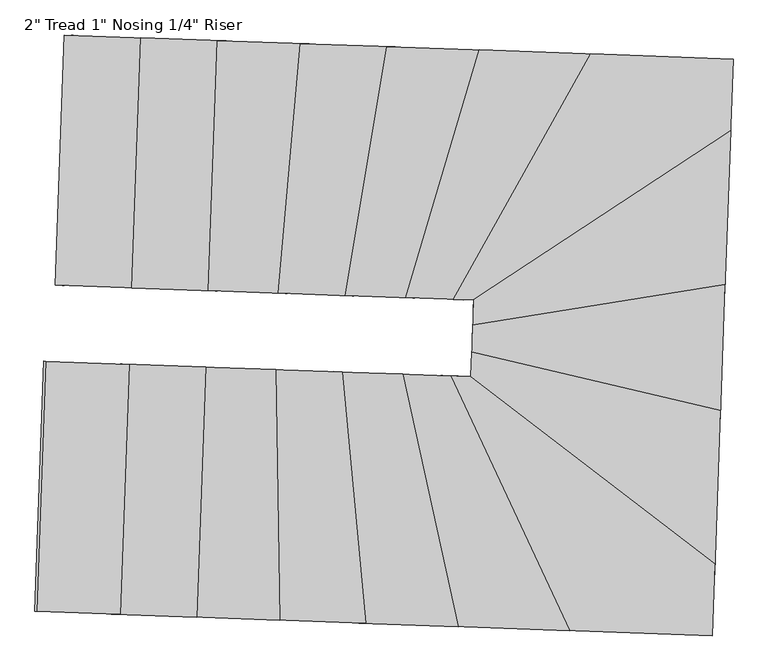
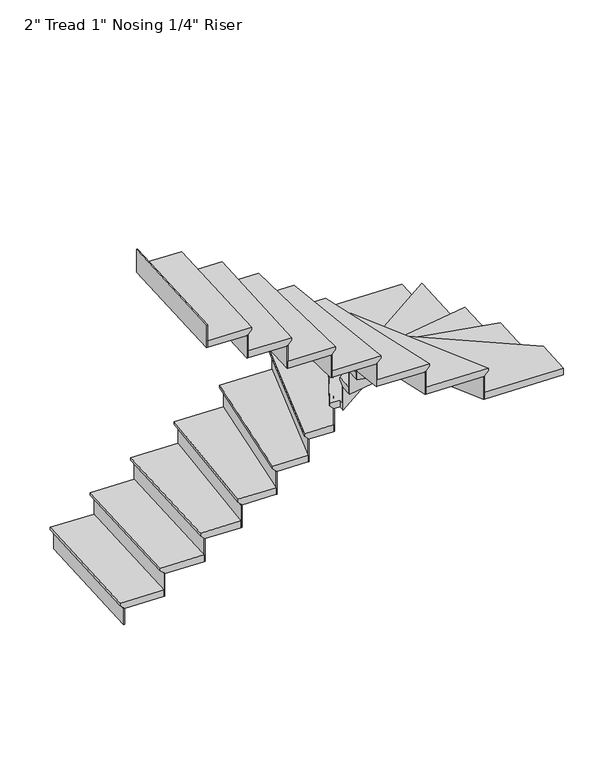
"""IFC4 building model written with IfcOpenShell, lengths in millimetres: stair flight geometry."""

from ifc_helpers import new_model, si_unit, origin, place, context, project, spatial, faceted_brep, source, transform, mapped, element, save


def stair_flight_664b5221(model_context):
    return source(origin(), model_context, "Body", "Brep", [
        faceted_brep([(-10039.2744432, -1277.1215258, 6246.2833333), (-10039.2744432, -1277.1215258, 6265.3333333), (-10006.394185, -363.3128759, 6265.3333333), (-10006.394185, -363.3128759, 6246.2833333), (-10013.8908696, -1278.0348663, 6220.8833333), (-9981.0106114, -364.2262164, 6220.8833333), (-9734.6715599, -1288.0816118, 6265.3333333), (-9701.7913017, -374.272962, 6265.3333333), (-9981.0106114, -364.2262164, 6214.5333333), (-9701.7913017, -374.272962, 6214.5333333), (-9734.6715599, -1288.0816118, 6214.5333333), (-10013.8908696, -1278.0348663, 6214.5333333)], [[[0, 1, 2, 3]], [[4, 0, 3, 5]], [[2, 1, 6, 7]], [[8, 9, 10, 11]], [[2, 7, 9, 8, 5, 3]], [[8, 11, 4, 5]], [[6, 1, 0, 4, 11, 10]], [[7, 6, 10, 9]]]),
        faceted_brep([(-10013.8908696, -1278.0348663, 6214.5333333), (-10013.8908696, -1278.0348663, 6096.0), (-10007.5449762, -1278.2632014, 6096.0), (-10007.5449762, -1278.2632014, 6214.5333333), (-9981.0106114, -364.2262164, 6214.5333333), (-9974.664718, -364.4545515, 6214.5333333), (-9974.664718, -364.4545515, 6096.0), (-9981.0106114, -364.2262164, 6096.0)], [[[0, 1, 2, 3]], [[4, 5, 6, 7]], [[1, 0, 4, 7]], [[2, 1, 7, 6]], [[3, 2, 6, 5]], [[0, 3, 5, 4]]]),
        faceted_brep([(-9734.6715599, -1288.0816118, 6383.8666667), (-9734.6715599, -1288.0816118, 6214.5333333), (-9728.3256665, -1288.309947, 6214.5333333), (-9728.3256665, -1288.309947, 6383.8666667), (-9701.7913017, -374.272962, 6383.8666667), (-9695.4454083, -374.5012971, 6383.8666667), (-9695.4454083, -374.5012971, 6214.5333333), (-9701.7913017, -374.272962, 6214.5333333)], [[[0, 1, 2, 3]], [[4, 5, 6, 7]], [[1, 0, 4, 7]], [[2, 1, 7, 6]], [[3, 2, 6, 5]], [[0, 3, 5, 4]]]),
        faceted_brep([(-9727.1748753, -373.3596215, 6434.6666667), (-9760.0551335, -1287.1682713, 6434.6666667), (-9455.4522502, -1298.1283574, 6434.6666667), (-9422.571992, -384.3197075, 6434.6666667), (-9701.7913017, -374.272962, 6383.8666667), (-9422.571992, -384.3197075, 6383.8666667), (-9455.4522502, -1298.1283574, 6383.8666667), (-9734.6715599, -1288.0816118, 6383.8666667), (-9701.7913017, -374.272962, 6390.2166667), (-9727.1748753, -373.3596215, 6415.6166667), (-9734.6715599, -1288.0816118, 6390.2166667), (-9760.0551335, -1287.1682713, 6415.6166667)], [[[0, 1, 2, 3]], [[4, 5, 6, 7]], [[0, 3, 5, 4, 8, 9]], [[4, 7, 10, 8]], [[2, 1, 11, 10, 7, 6]], [[3, 2, 6, 5]], [[11, 1, 0, 9]], [[10, 11, 9, 8]]]),
        faceted_brep([(-9455.4522502, -1298.1283574, 6553.2), (-9455.4522502, -1298.1283574, 6383.8666667), (-9449.1063568, -1298.3566925, 6383.8666667), (-9449.1063568, -1298.3566925, 6553.2), (-9422.571992, -384.3197075, 6553.2), (-9416.2260986, -384.5480426, 6553.2), (-9416.2260986, -384.5480426, 6383.8666667), (-9422.571992, -384.3197075, 6383.8666667)], [[[0, 1, 2, 3]], [[4, 5, 6, 7]], [[1, 0, 4, 7]], [[2, 1, 7, 6]], [[3, 2, 6, 5]], [[0, 3, 5, 4]]]),
        faceted_brep([(-9447.9555656, -383.406367, 6604.0), (-9480.8358238, -1297.2150169, 6604.0), (-9199.9504308, -1307.3217107, 6604.0), (-9119.566643, -395.2223118, 6604.0), (-9422.571992, -384.3197075, 6553.2), (-9119.566643, -395.2223118, 6553.2), (-9199.9504308, -1307.3217107, 6553.2), (-9455.4522502, -1298.1283574, 6553.2), (-9422.571992, -384.3197075, 6559.55), (-9447.9555656, -383.406367, 6584.95), (-9455.4522502, -1298.1283574, 6559.55), (-9480.8358238, -1297.2150169, 6584.95)], [[[0, 1, 2, 3]], [[4, 5, 6, 7]], [[0, 3, 5, 4, 8, 9]], [[4, 7, 10, 8]], [[2, 1, 11, 10, 7, 6]], [[3, 2, 6, 5]], [[11, 1, 0, 9]], [[10, 11, 9, 8]]]),
        faceted_brep([(-9199.9504308, -1307.3217107, 6722.5333333), (-9199.9504308, -1307.3217107, 6553.2), (-9193.5959688, -1307.5503542, 6553.2), (-9193.5959688, -1307.5503542, 6722.5333333), (-9119.566643, -395.2223118, 6722.5333333), (-9113.212181, -395.4509552, 6722.5333333), (-9113.212181, -395.4509552, 6553.2), (-9119.566643, -395.2223118, 6553.2)], [[[0, 1, 2, 3]], [[4, 5, 6, 7]], [[1, 0, 4, 7]], [[2, 1, 7, 6]], [[3, 2, 6, 5]], [[0, 3, 5, 4]]]),
        faceted_brep([(-9144.9844911, -394.3077381, 6773.3333333), (-9225.3682789, -1306.407137, 6773.3333333), (-8955.9416356, -1316.1015272, 6773.3333333), (-8804.7818676, -406.5487582, 6773.3333333), (-9119.566643, -395.2223118, 6722.5333333), (-8804.7818676, -406.5487582, 6722.5333333), (-8955.9416356, -1316.1015272, 6722.5333333), (-9199.9504308, -1307.3217107, 6722.5333333), (-9119.566643, -395.2223118, 6728.8833333), (-9144.9844911, -394.3077381, 6754.2833333), (-9199.9504308, -1307.3217107, 6728.8833333), (-9225.3682789, -1306.407137, 6754.2833333)], [[[0, 1, 2, 3]], [[4, 5, 6, 7]], [[0, 3, 5, 4, 8, 9]], [[4, 7, 10, 8]], [[2, 1, 11, 10, 7, 6]], [[3, 2, 6, 5]], [[11, 1, 0, 9]], [[10, 11, 9, 8]]]),
        faceted_brep([(-8955.9416356, -1316.1015272, 6891.8666667), (-8955.9416356, -1316.1015272, 6722.5333333), (-8949.5428047, -1316.3317671, 6722.5333333), (-8949.5428047, -1316.3317671, 6891.8666667), (-8804.7818676, -406.5487582, 6891.8666667), (-8798.3830367, -406.7789981, 6891.8666667), (-8798.3830367, -406.7789981, 6722.5333333), (-8804.7818676, -406.5487582, 6722.5333333)], [[[0, 1, 2, 3]], [[4, 5, 6, 7]], [[1, 0, 4, 7]], [[2, 1, 7, 6]], [[3, 2, 6, 5]], [[0, 3, 5, 4]]]),
        faceted_brep([(-8830.3771913, -405.6277986, 6942.6666667), (-8981.5369593, -1315.1805676, 6942.6666667), (-8734.4577413, -1324.0708626, 6942.6666667), (-8466.5990966, -418.7171009, 6942.6666667), (-8804.7818676, -406.5487582, 6891.8666667), (-8466.5990966, -418.7171009, 6891.8666667), (-8734.4577413, -1324.0708626, 6891.8666667), (-8955.9416356, -1316.1015272, 6891.8666667), (-8804.7818676, -406.5487582, 6898.2166667), (-8830.3771913, -405.6277986, 6923.6166667), (-8955.9416356, -1316.1015272, 6898.2166667), (-8981.5369593, -1315.1805676, 6923.6166667)], [[[0, 1, 2, 3]], [[4, 5, 6, 7]], [[0, 3, 5, 4, 8, 9]], [[4, 7, 10, 8]], [[2, 1, 11, 10, 7, 6]], [[3, 2, 6, 5]], [[11, 1, 0, 9]], [[10, 11, 9, 8]]]),
        faceted_brep([(-8734.4577413, -1324.0708626, 7061.2), (-8734.4577413, -1324.0708626, 6891.8666667), (-8727.9054047, -1324.3066258, 6891.8666667), (-8727.9054047, -1324.3066258, 7061.2), (-8466.5990966, -418.7171009, 7061.2), (-8460.0467599, -418.9528642, 7061.2), (-8460.0467599, -418.9528642, 6891.8666667), (-8466.5990966, -418.7171009, 6891.8666667)], [[[0, 1, 2, 3]], [[4, 5, 6, 7]], [[1, 0, 4, 7]], [[2, 1, 7, 6]], [[3, 2, 6, 5]], [[0, 3, 5, 4]]]),
        faceted_brep([(-8492.8084432, -417.7740478, 7112.0), (-8760.667088, -1323.1278095, 7112.0), (-8558.2251501, -1330.4119856, 7112.0), (-8056.8234634, -433.4614663, 7112.0), (-8466.5990966, -418.7171009, 7061.2), (-8056.8234634, -433.4614663, 7061.2), (-8558.2251501, -1330.4119856, 7061.2), (-8734.4577413, -1324.0708626, 7061.2), (-8466.5990966, -418.7171009, 7067.55), (-8492.8084432, -417.7740478, 7092.95), (-8734.4577413, -1324.0708626, 7067.55), (-8760.667088, -1323.1278095, 7092.95)], [[[0, 1, 2, 3]], [[4, 5, 6, 7]], [[0, 3, 5, 4, 8, 9]], [[4, 7, 10, 8]], [[2, 1, 11, 10, 7, 6]], [[3, 2, 6, 5]], [[11, 1, 0, 9]], [[10, 11, 9, 8]]]),
        faceted_brep([(-8558.2251501, -1330.4119856, 7230.5333333), (-8558.2251501, -1330.4119856, 7061.2), (-8551.0937819, -1330.6685834, 7061.2), (-8551.0937819, -1330.6685834, 7230.5333333), (-8056.8234634, -433.4614663, 7230.5333333), (-8049.6920951, -433.718064, 7230.5333333), (-8049.6920951, -433.718064, 7061.2), (-8056.8234634, -433.4614663, 7061.2)], [[[0, 1, 2, 3]], [[4, 5, 6, 7]], [[1, 0, 4, 7]], [[2, 1, 7, 6]], [[3, 2, 6, 5]], [[0, 3, 5, 4]]]),
        faceted_brep([(-7576.4021107, -744.6189573, 7281.3333333), (-7565.8418401, -451.1277497, 7281.3333333), (-8085.3489363, -432.4350754, 7281.3333333), (-8586.750623, -1329.3855947, 7281.3333333), (-8512.5307482, -1332.0561414, 7281.3333333), (-8513.5934983, -1361.5921107, 7281.3333333), (-7565.8418401, -451.1277497, 7230.5333333), (-7576.4021107, -744.6189573, 7230.5333333), (-8513.5934983, -1361.5921107, 7230.5333333), (-8512.5307482, -1332.0561414, 7230.5333333), (-8558.2251501, -1330.4119856, 7230.5333333), (-8056.8234634, -433.4614663, 7230.5333333), (-8056.8234634, -433.4614663, 7236.8833333), (-8085.3489363, -432.4350754, 7262.2833333), (-8558.2251501, -1330.4119856, 7236.8833333), (-8586.750623, -1329.3855947, 7262.2833333)], [[[0, 1, 2, 3, 4, 5]], [[6, 7, 8, 9, 10, 11]], [[1, 0, 7, 6]], [[2, 1, 6, 11, 12, 13]], [[11, 10, 14, 12]], [[4, 3, 15, 14, 10, 9]], [[5, 4, 9, 8]], [[0, 5, 8, 7]], [[15, 3, 2, 13]], [[14, 15, 13, 12]]]),
        faceted_brep([(-8513.5934983, -1361.5921107, 7399.8666667), (-8513.5934983, -1361.5921107, 7230.5333333), (-8513.8736844, -1369.3790464, 7230.5333333), (-8513.8736844, -1369.3790464, 7399.8666667), (-7576.4021107, -744.6189573, 7399.8666667), (-7576.6822968, -752.405893, 7399.8666667), (-7576.6822968, -752.405893, 7230.5333333), (-7576.4021107, -744.6189573, 7230.5333333)], [[[0, 1, 2, 3]], [[4, 5, 6, 7]], [[1, 0, 4, 7]], [[2, 1, 7, 6]], [[3, 2, 6, 5]], [[0, 3, 5, 4]]]),
        faceted_brep([(-7575.2813665, -713.4712147, 7450.6666667), (-8512.472754, -1330.4443681, 7450.6666667), (-8516.7022393, -1447.9902872, 7450.6666667), (-7596.4124368, -1300.7462523, 7450.6666667), (-7576.4021107, -744.6189573, 7399.8666667), (-7596.4124368, -1300.7462523, 7399.8666667), (-8516.7022393, -1447.9902872, 7399.8666667), (-8513.5934983, -1361.5921107, 7399.8666667), (-7576.4021107, -744.6189573, 7406.2166667), (-7575.2813665, -713.4712147, 7431.6166667), (-8513.5934983, -1361.5921107, 7406.2166667), (-8512.472754, -1330.4443681, 7431.6166667)], [[[0, 1, 2, 3]], [[4, 5, 6, 7]], [[0, 3, 5, 4, 8, 9]], [[4, 7, 10, 8]], [[2, 1, 11, 10, 7, 6]], [[3, 2, 6, 5]], [[11, 1, 0, 9]], [[10, 11, 9, 8]]]),
        faceted_brep([(-8516.7022393, -1447.9902872, 7569.2), (-8516.7022393, -1447.9902872, 7399.8666667), (-8516.934968, -1454.458287, 7399.8666667), (-8516.934968, -1454.458287, 7569.2), (-7596.4124368, -1300.7462523, 7569.2), (-7596.6451655, -1307.2142521, 7569.2), (-7596.6451655, -1307.2142521, 7399.8666667), (-7596.4124368, -1300.7462523, 7399.8666667)], [[[0, 1, 2, 3]], [[4, 5, 6, 7]], [[1, 0, 4, 7]], [[2, 1, 7, 6]], [[3, 2, 6, 5]], [[0, 3, 5, 4]]]),
        faceted_brep([(-7595.481522, -1274.874253, 7620.0), (-8515.7713244, -1422.1182879, 7620.0), (-8520.2678323, -1547.0853038, 7620.0), (-7612.9403349, -1760.0898551, 7620.0), (-7596.4124368, -1300.7462523, 7569.2), (-7612.9403349, -1760.0898551, 7569.2), (-8520.2678323, -1547.0853038, 7569.2), (-8516.7022393, -1447.9902872, 7569.2), (-7596.4124368, -1300.7462523, 7575.55), (-7595.481522, -1274.874253, 7600.95), (-8516.7022393, -1447.9902872, 7575.55), (-8515.7713244, -1422.1182879, 7600.95)], [[[0, 1, 2, 3]], [[4, 5, 6, 7]], [[0, 3, 5, 4, 8, 9]], [[4, 7, 10, 8]], [[2, 1, 11, 10, 7, 6]], [[3, 2, 6, 5]], [[11, 1, 0, 9]], [[10, 11, 9, 8]]]),
        faceted_brep([(-8520.2678323, -1547.0853038, 7738.5333333), (-8520.2678323, -1547.0853038, 7569.2), (-8520.500561, -1553.5533036, 7569.2), (-8520.500561, -1553.5533036, 7738.5333333), (-7612.9403349, -1760.0898551, 7738.5333333), (-7613.1730636, -1766.5578549, 7738.5333333), (-7613.1730636, -1766.5578549, 7569.2), (-7612.9403349, -1760.0898551, 7569.2)], [[[0, 1, 2, 3]], [[4, 5, 6, 7]], [[1, 0, 4, 7]], [[2, 1, 7, 6]], [[3, 2, 6, 5]], [[0, 3, 5, 4]]]),
        faceted_brep([(-7612.0094201, -1734.2178558, 7789.3333333), (-8519.3369174, -1521.2133045, 7789.3333333), (-8522.5774937, -1611.2754511, 7789.3333333), (-8568.6431579, -1609.6179367, 7789.3333333), (-7633.3303199, -2326.7686368, 7789.3333333), (-7612.9403349, -1760.0898551, 7738.5333333), (-7633.3303199, -2326.7686368, 7738.5333333), (-8568.6431579, -1609.6179367, 7738.5333333), (-8522.5774937, -1611.2754511, 7738.5333333), (-8520.2678323, -1547.0853038, 7738.5333333), (-7612.9403349, -1760.0898551, 7744.8833333), (-7612.0094201, -1734.2178558, 7770.2833333), (-8520.2678323, -1547.0853038, 7744.8833333), (-8519.3369174, -1521.2133045, 7770.2833333)], [[[0, 1, 2, 3, 4]], [[5, 6, 7, 8, 9]], [[0, 4, 6, 5, 10, 11]], [[5, 9, 12, 10]], [[2, 1, 13, 12, 9, 8]], [[3, 2, 8, 7]], [[4, 3, 7, 6]], [[13, 1, 0, 11]], [[12, 13, 11, 10]]]),
        faceted_brep([(-8568.6431579, -1609.6179367, 7907.8666667), (-8568.6431579, -1609.6179367, 7738.5333333), (-8579.5929645, -1609.2239456, 7738.5333333), (-8579.5929645, -1609.2239456, 7907.8666667), (-7633.3303199, -2326.7686368, 7907.8666667), (-7633.610506, -2334.5555724, 7907.8666667), (-7633.610506, -2334.5555724, 7738.5333333), (-7633.3303199, -2326.7686368, 7738.5333333)], [[[0, 1, 2, 3]], [[4, 5, 6, 7]], [[1, 0, 4, 7]], [[2, 1, 7, 6]], [[3, 2, 6, 5]], [[0, 3, 5, 4]]]),
        faceted_brep([(-8189.6816712, -2538.2452939, 7958.6666667), (-7641.649102, -2557.9643591, 7958.6666667), (-7632.2095756, -2295.6208941, 7958.6666667), (-8524.8439316, -1611.1939011, 7958.6666667), (-8625.3228415, -1607.5785134, 7958.6666667), (-7641.649102, -2557.9643591, 7907.8666667), (-8189.6816712, -2538.2452939, 7907.8666667), (-8625.3228415, -1607.5785134, 7907.8666667), (-8568.6431579, -1609.6179367, 7907.8666667), (-7633.3303199, -2326.7686368, 7907.8666667), (-7633.3303199, -2326.7686368, 7914.2166667), (-7632.2095756, -2295.6208941, 7939.6166667), (-8568.6431579, -1609.6179367, 7914.2166667), (-8524.8439316, -1611.1939011, 7939.6166667)], [[[0, 1, 2, 3, 4]], [[5, 6, 7, 8, 9]], [[1, 0, 6, 5]], [[2, 1, 5, 9, 10, 11]], [[9, 8, 12, 10]], [[4, 3, 13, 12, 8, 7]], [[0, 4, 7, 6]], [[13, 3, 2, 11]], [[12, 13, 11, 10]]]),
        faceted_brep([(-8625.3228415, -1607.5785134, 8077.2), (-8625.3228415, -1607.5785134, 7907.8666667), (-8632.4542098, -1607.3219157, 7907.8666667), (-8632.4542098, -1607.3219157, 8077.2), (-8189.6816712, -2538.2452939, 8077.2), (-8196.8130394, -2537.9886962, 8077.2), (-8196.8130394, -2537.9886962, 7907.8666667), (-8189.6816712, -2538.2452939, 7907.8666667)], [[[0, 1, 2, 3]], [[4, 5, 6, 7]], [[1, 0, 4, 7]], [[2, 1, 7, 6]], [[3, 2, 6, 5]], [[0, 3, 5, 4]]]),
        faceted_brep([(-8161.1561983, -2539.2716849, 8128.0), (-8596.7973686, -1608.6049044, 8128.0), (-8796.9231803, -1601.404066, 8128.0), (-8594.8250519, -2523.6676042, 8128.0), (-8189.6816712, -2538.2452939, 8077.2), (-8594.8250519, -2523.6676042, 8077.2), (-8796.9231803, -1601.404066, 8077.2), (-8625.3228415, -1607.5785134, 8077.2), (-8189.6816712, -2538.2452939, 8083.55), (-8161.1561983, -2539.2716849, 8108.95), (-8625.3228415, -1607.5785134, 8083.55), (-8596.7973686, -1608.6049044, 8108.95)], [[[0, 1, 2, 3]], [[4, 5, 6, 7]], [[0, 3, 5, 4, 8, 9]], [[4, 7, 10, 8]], [[2, 1, 11, 10, 7, 6]], [[3, 2, 6, 5]], [[11, 1, 0, 9]], [[10, 11, 9, 8]]]),
        faceted_brep([(-8796.9231803, -1601.404066, 8246.5333333), (-8796.9231803, -1601.404066, 8077.2), (-8803.475517, -1601.1683028, 8077.2), (-8803.475517, -1601.1683028, 8246.5333333), (-8594.8250519, -2523.6676042, 8246.5333333), (-8601.3773886, -2523.4318409, 8246.5333333), (-8601.3773886, -2523.4318409, 8077.2), (-8594.8250519, -2523.6676042, 8077.2)], [[[0, 1, 2, 3]], [[4, 5, 6, 7]], [[1, 0, 4, 7]], [[2, 1, 7, 6]], [[3, 2, 6, 5]], [[0, 3, 5, 4]]]),
        faceted_brep([(-8568.6157052, -2524.6106573, 8297.3333333), (-8770.7138336, -1602.3471191, 8297.3333333), (-9017.1790286, -1593.4789176, 8297.3333333), (-8931.779777, -2511.5434485, 8297.3333333), (-8594.8250519, -2523.6676042, 8246.5333333), (-8931.779777, -2511.5434485, 8246.5333333), (-9017.1790286, -1593.4789176, 8246.5333333), (-8796.9231803, -1601.404066, 8246.5333333), (-8594.8250519, -2523.6676042, 8252.8833333), (-8568.6157052, -2524.6106573, 8278.2833333), (-8796.9231803, -1601.404066, 8252.8833333), (-8770.7138336, -1602.3471191, 8278.2833333)], [[[0, 1, 2, 3]], [[4, 5, 6, 7]], [[0, 3, 5, 4, 8, 9]], [[4, 7, 10, 8]], [[2, 1, 11, 10, 7, 6]], [[3, 2, 6, 5]], [[11, 1, 0, 9]], [[10, 11, 9, 8]]]),
        faceted_brep([(-9017.1790286, -1593.4789176, 8415.8666667), (-9017.1790286, -1593.4789176, 8246.5333333), (-9023.5778595, -1593.2486777, 8246.5333333), (-9023.5778595, -1593.2486777, 8415.8666667), (-8931.779777, -2511.5434485, 8415.8666667), (-8938.1786079, -2511.3132086, 8415.8666667), (-8938.1786079, -2511.3132086, 8246.5333333), (-8931.779777, -2511.5434485, 8246.5333333)], [[[0, 1, 2, 3]], [[4, 5, 6, 7]], [[1, 0, 4, 7]], [[2, 1, 7, 6]], [[3, 2, 6, 5]], [[0, 3, 5, 4]]]),
        faceted_brep([(-8906.1844533, -2512.4644081, 8466.6666667), (-8991.5837049, -1594.3998772, 8466.6666667), (-9260.8328726, -1584.7118729, 8466.6666667), (-9246.2096012, -2500.2297738, 8466.6666667), (-8931.779777, -2511.5434485, 8415.8666667), (-9246.2096012, -2500.2297738, 8415.8666667), (-9260.8328726, -1584.7118729, 8415.8666667), (-9017.1790286, -1593.4789176, 8415.8666667), (-8931.779777, -2511.5434485, 8422.2166667), (-8906.1844533, -2512.4644081, 8447.6166667), (-9017.1790286, -1593.4789176, 8422.2166667), (-8991.5837049, -1594.3998772, 8447.6166667)], [[[0, 1, 2, 3]], [[4, 5, 6, 7]], [[0, 3, 5, 4, 8, 9]], [[4, 7, 10, 8]], [[2, 1, 11, 10, 7, 6]], [[3, 2, 6, 5]], [[11, 1, 0, 9]], [[10, 11, 9, 8]]]),
        faceted_brep([(-9260.8328726, -1584.7118729, 8585.2), (-9260.8328726, -1584.7118729, 8415.8666667), (-9267.1873346, -1584.4832295, 8415.8666667), (-9267.1873346, -1584.4832295, 8585.2), (-9246.2096012, -2500.2297738, 8585.2), (-9252.5640632, -2500.0011303, 8585.2), (-9252.5640632, -2500.0011303, 8415.8666667), (-9246.2096012, -2500.2297738, 8415.8666667)], [[[0, 1, 2, 3]], [[4, 5, 6, 7]], [[1, 0, 4, 7]], [[2, 1, 7, 6]], [[3, 2, 6, 5]], [[0, 3, 5, 4]]]),
        faceted_brep([(-9220.7917531, -2501.1443475, 8636.0), (-9235.4150245, -1585.6264467, 8636.0), (-9516.266143, -1575.5209861, 8636.0), (-9549.1464012, -2489.329636, 8636.0), (-9246.2096012, -2500.2297738, 8585.2), (-9549.1464012, -2489.329636, 8585.2), (-9516.266143, -1575.5209861, 8585.2), (-9260.8328726, -1584.7118729, 8585.2), (-9246.2096012, -2500.2297738, 8591.55), (-9220.7917531, -2501.1443475, 8616.95), (-9260.8328726, -1584.7118729, 8591.55), (-9235.4150245, -1585.6264467, 8616.95)], [[[0, 1, 2, 3]], [[4, 5, 6, 7]], [[0, 3, 5, 4, 8, 9]], [[4, 7, 10, 8]], [[2, 1, 11, 10, 7, 6]], [[3, 2, 6, 5]], [[11, 1, 0, 9]], [[10, 11, 9, 8]]]),
        faceted_brep([(-9516.266143, -1575.5209861, 8754.5333333), (-9516.266143, -1575.5209861, 8585.2), (-9522.6120364, -1575.292651, 8585.2), (-9522.6120364, -1575.292651, 8754.5333333), (-9549.1464012, -2489.329636, 8754.5333333), (-9555.4922946, -2489.1013009, 8754.5333333), (-9555.4922946, -2489.1013009, 8585.2), (-9549.1464012, -2489.329636, 8585.2)], [[[0, 1, 2, 3]], [[4, 5, 6, 7]], [[1, 0, 4, 7]], [[2, 1, 7, 6]], [[3, 2, 6, 5]], [[0, 3, 5, 4]]]),
        faceted_brep([(-9523.7628276, -2490.2429765, 8805.3333333), (-9490.8825694, -1576.4343266, 8805.3333333), (-9795.4854527, -1565.4742405, 8805.3333333), (-9828.3657109, -2479.2828904, 8805.3333333), (-9549.1464012, -2489.329636, 8754.5333333), (-9828.3657109, -2479.2828904, 8754.5333333), (-9795.4854527, -1565.4742405, 8754.5333333), (-9516.266143, -1575.5209861, 8754.5333333), (-9549.1464012, -2489.329636, 8760.8833333), (-9523.7628276, -2490.2429765, 8786.2833333), (-9516.266143, -1575.5209861, 8760.8833333), (-9490.8825694, -1576.4343266, 8786.2833333)], [[[0, 1, 2, 3]], [[4, 5, 6, 7]], [[0, 3, 5, 4, 8, 9]], [[4, 7, 10, 8]], [[2, 1, 11, 10, 7, 6]], [[3, 2, 6, 5]], [[11, 1, 0, 9]], [[10, 11, 9, 8]]]),
        faceted_brep([(-9795.4854527, -1565.4742405, 8923.8666667), (-9795.4854527, -1565.4742405, 8754.5333333), (-9801.8313461, -1565.2459054, 8754.5333333), (-9801.8313461, -1565.2459054, 8923.8666667), (-9828.3657109, -2479.2828904, 8923.8666667), (-9834.7116043, -2479.0545553, 8923.8666667), (-9834.7116043, -2479.0545553, 8754.5333333), (-9828.3657109, -2479.2828904, 8754.5333333)], [[[0, 1, 2, 3]], [[4, 5, 6, 7]], [[1, 0, 4, 7]], [[2, 1, 7, 6]], [[3, 2, 6, 5]], [[0, 3, 5, 4]]]),
        faceted_brep([(-10074.7047624, -1555.427495, 9093.2), (-10074.7047624, -1555.427495, 8923.8666667), (-10081.0506558, -1555.1991598, 8923.8666667), (-10081.0506558, -1555.1991598, 9093.2), (-10107.5850206, -2469.2361449, 9093.2), (-10113.930914, -2469.0078097, 9093.2), (-10113.930914, -2469.0078097, 8923.8666667), (-10107.5850206, -2469.2361449, 8923.8666667)], [[[0, 1, 2, 3]], [[4, 5, 6, 7]], [[1, 0, 4, 7]], [[2, 1, 7, 6]], [[3, 2, 6, 5]], [[0, 3, 5, 4]]]),
        faceted_brep([(-9802.9821373, -2480.1962309, 8974.6666667), (-9770.1018791, -1566.387581, 8974.6666667), (-10074.7047624, -1555.427495, 8974.6666667), (-10107.5850206, -2469.2361449, 8974.6666667), (-9828.3657109, -2479.2828904, 8923.8666667), (-10107.5850206, -2469.2361449, 8923.8666667), (-10074.7047624, -1555.427495, 8923.8666667), (-9795.4854527, -1565.4742405, 8923.8666667), (-9828.3657109, -2479.2828904, 8930.2166667), (-9802.9821373, -2480.1962309, 8955.6166667), (-9795.4854527, -1565.4742405, 8930.2166667), (-9770.1018791, -1566.387581, 8955.6166667)], [[[0, 1, 2, 3]], [[4, 5, 6, 7]], [[0, 3, 5, 4, 8, 9]], [[4, 7, 10, 8]], [[2, 1, 11, 10, 7, 6]], [[3, 2, 6, 5]], [[11, 1, 0, 9]], [[10, 11, 9, 8]]]),
    ])


if __name__ == "__main__":
    model = new_model("IFC4")
    model_context = context("Model", 3, world=origin())
    ifc_project = project(units=[si_unit("LENGTHUNIT", "METRE", prefix="MILLI")], contexts=[model_context])
    site = spatial("IfcSite", under=ifc_project)
    building = spatial("IfcBuilding", under=site)
    placement = place(None, origin())
    stair_flight_shape = stair_flight_664b5221(model_context)
    element("IfcStairFlight", 1, ObjectType="2\" Tread 1\" Nosing 1/4\" Riser", at=placement, inside=building, context=model_context, shape_type="MappedRepresentation", body=[
        mapped(stair_flight_shape, transform((0.0, 0.0, 0.0), x_axis=(1.0, 0.0, 0.0), y_axis=(0.0, 1.0, 0.0), z_axis=(0.0, 0.0, 1.0))),
    ])
    save(model, "model.ifc")

# Revit data of these elements
# Element 1 (IfcStairFlight, "2\" Tread 1\" Nosing 1/4\" Riser")
#   Materials on its faces: "Cherry"
# Materials
#   "Cherry": class "Wood", colour RGB 226 177 128, transparency 0, Description = "Prunus Serotina", Cost = 0
